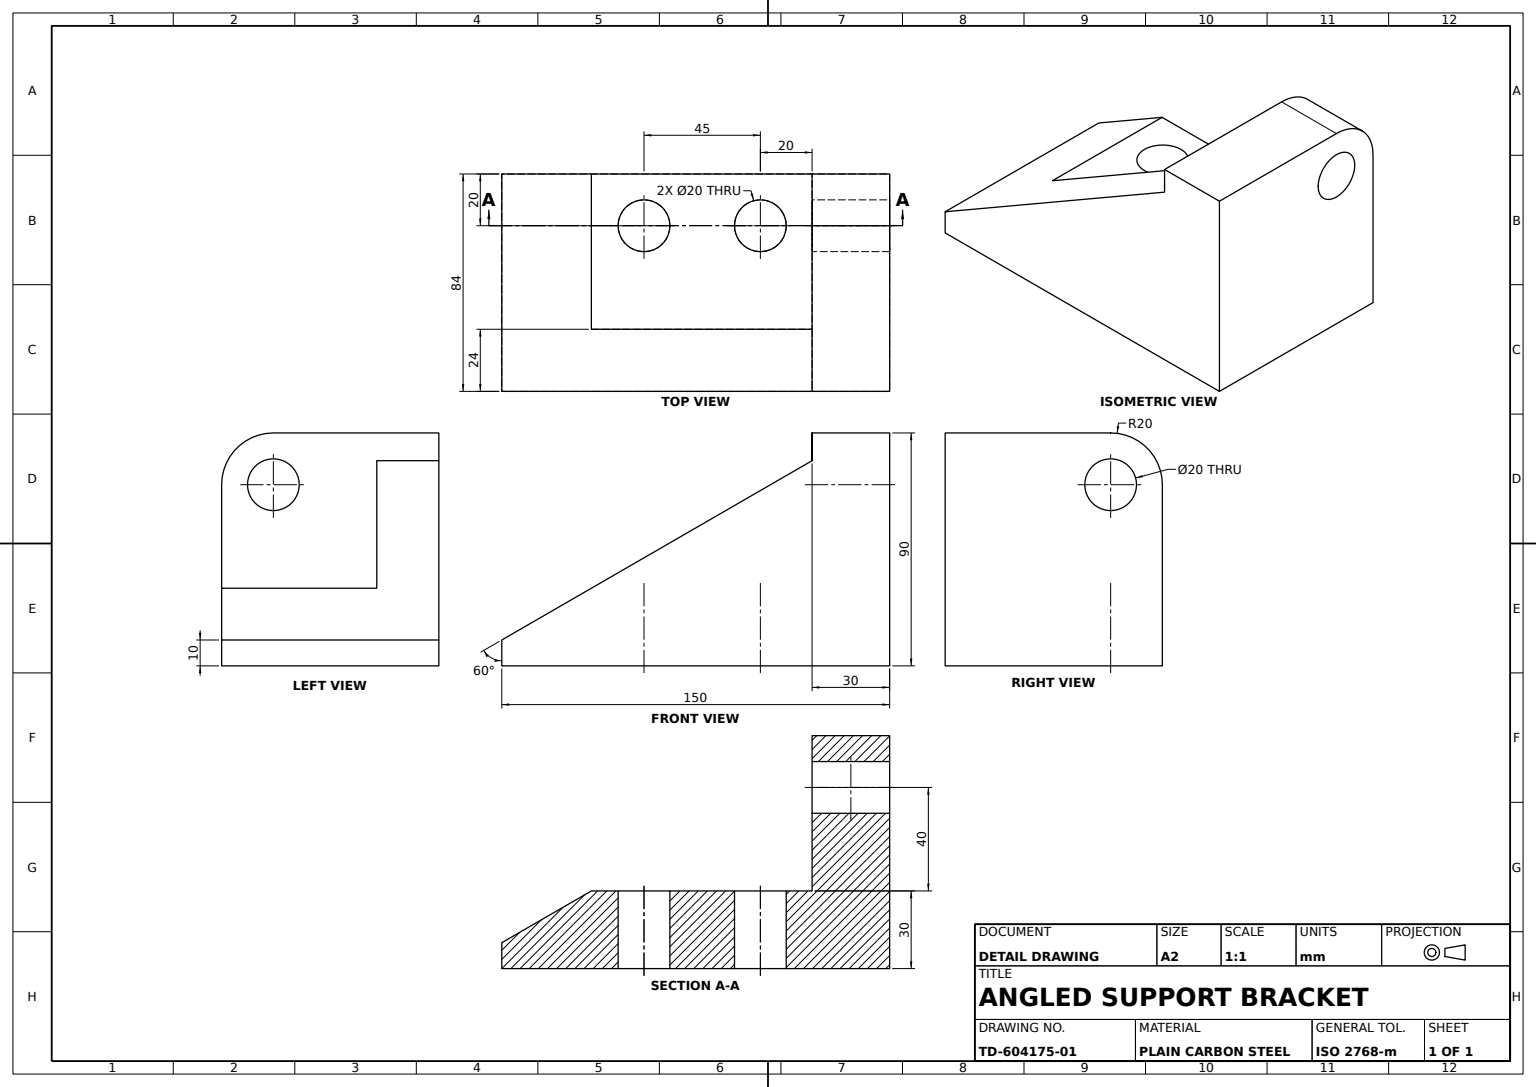
from build123d import *

# Parameters (mm, degrees)
BRACKET_BODY_DEPTH     = 84
GUSSET_DEPTH           = 24
BASE_HOLES_SKETCH_R    = 10
BASE_HOLES_2X_20_DEPTH = 30
LUG_HOLE_SKETCH_R      = 10
LUG_HOLE_20_DEPTH      = 208
LUG_TOP_FILLET_R20_R   = 20


with BuildPart() as part:
    # Bracket Profile Sketch → Bracket Body (new body)
    with BuildSketch(Plane(origin=(0, 0, 0), x_dir=(0, 0, -1), z_dir=(1, 0, 0))):
        Polygon((0, 10), (0, 0), (150, 0), (150, 90), (120, 90), (120, 79.282032303), (120, 70), (120, 30), (34.641016151, 30), align=None)
    extrude(amount=-BRACKET_BODY_DEPTH)

    # Gusset Sketch → Gusset (add)
    with BuildSketch(Plane(origin=(0, 0, 0), x_dir=(0, 0, -1), z_dir=(1, 0, 0))):
        Polygon((34.641016151, 30), (120, 79.282032303), (120, 30), align=None)
    extrude(amount=-GUSSET_DEPTH)

    # Base Holes Sketch → Base Holes 2xØ20 (cut)
    with BuildSketch(Plane(origin=(0, 0, 0), x_dir=(1, 0, 0), z_dir=(0, 1, 0))):
        with Locations(Location((-64, 100, 0), (0, 0, 270))):
            Circle(BASE_HOLES_SKETCH_R)
        with Locations(Location((-64, 55, 0), (0, 0, 270))):
            Circle(BASE_HOLES_SKETCH_R)
    extrude(amount=BASE_HOLES_2X_20_DEPTH, mode=Mode.SUBTRACT)

    # Lug Hole Sketch → Lug Hole Ø20 (cut)
    with BuildSketch(Plane.XY):
        with Locations((-64, 70)):
            Circle(LUG_HOLE_SKETCH_R)
    extrude(amount=-LUG_HOLE_20_DEPTH, mode=Mode.SUBTRACT)

    # Lug Top Fillet R20
    lug_top_fillet_r20_edges = [part.edges().sort_by_distance(p)[0] for p in [
        (-84, 90, -135),
    ]]
    fillet(lug_top_fillet_r20_edges, radius=LUG_TOP_FILLET_R20_R)


solid = part.part
